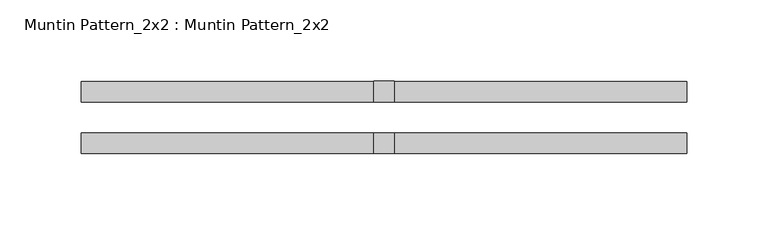
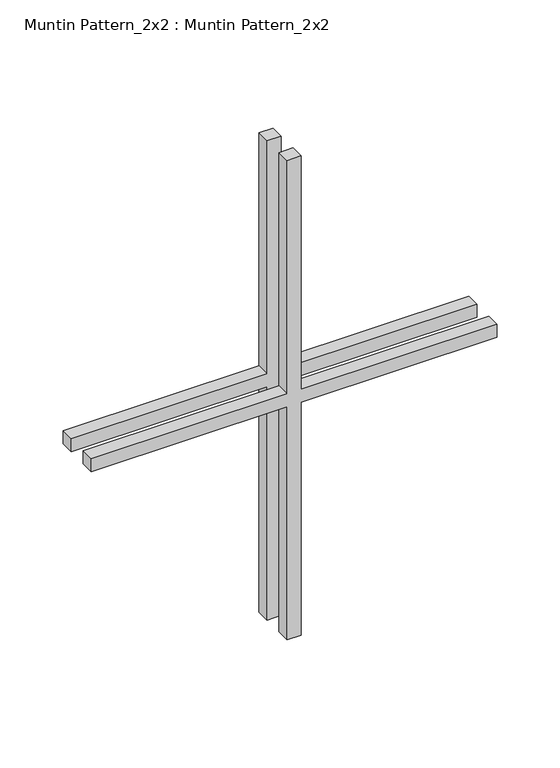
"""IFC4 building model written with IfcOpenShell, lengths in millimetres: proxy geometry, Muntin Pattern_2x2 : Muntin Pattern_2x2."""

from ifc_helpers import new_model, si_unit, frame, origin, place, context, project, spatial, polyline, outline, extrude, source, transform, mapped, element, save


def muntin_pattern_2x2_muntin_pattern_2x2_87da473c(model_context):
    return source(origin(), model_context, "Body", "SweptSolid", [
        extrude(outline(polyline([(238.125, -6.35), (238.125, -185.7375), (225.425, -185.7375), (225.425, -6.35), (0.0, -6.35), (0.0, 6.35), (225.425, 6.35), (225.425, 185.7375), (238.125, 185.7375), (238.125, 6.35), (463.55, 6.35), (463.55, -6.35), (238.125, -6.35)])), frame((0.0, 9.525, 0.0), z_axis=(0.0, 1.0, 0.0), x_axis=(0.0, 0.0, 1.0)), (0.0, 0.0, 1.0), 12.7),
        extrude(outline(polyline([(238.125, -6.35), (238.125, -185.7375), (225.425, -185.7375), (225.425, -6.35), (0.0, -6.35), (0.0, 6.35), (225.425, 6.35), (225.425, 185.7375), (238.125, 185.7375), (238.125, 6.35), (463.55, 6.35), (463.55, -6.35), (238.125, -6.35)])), frame((0.0, -22.225, 0.0), z_axis=(0.0, 1.0, 0.0), x_axis=(0.0, 0.0, 1.0)), (0.0, 0.0, 1.0), 12.7),
    ])


if __name__ == "__main__":
    model = new_model("IFC4")
    model_context = context("Model", 3, world=origin())
    ifc_project = project(units=[si_unit("LENGTHUNIT", "METRE", prefix="MILLI")], contexts=[model_context])
    site = spatial("IfcSite", under=ifc_project)
    building = spatial("IfcBuilding", under=site)
    placement = place(None, origin())
    muntin_pattern_2x2_muntin_pattern_2x2_shape = muntin_pattern_2x2_muntin_pattern_2x2_87da473c(model_context)
    element("IfcBuildingElementProxy", 1, Name="Muntin Pattern_2x2 : Muntin Pattern_2x2", ObjectType="Muntin Pattern_2x2 : Muntin Pattern_2x2", at=placement, inside=building, context=model_context, shape_type="MappedRepresentation", body=[
        mapped(muntin_pattern_2x2_muntin_pattern_2x2_shape, transform((0.0, 0.0, 0.0), x_axis=(1.0, 0.0, 0.0), y_axis=(0.0, 1.0, 0.0), z_axis=(0.0, 0.0, 1.0))),
    ])
    save(model, "model.ifc")

# Revit data of these elements
# Type "Muntin Pattern_2x2 : Muntin Pattern_2x2"
#   Width [instance default] = 4' - 0"
#   Thickness = 0' - 0 1/2"
#   Height [instance default] = 4' - 0"
#   Distance = 0' - 0 3/4"
#   Interior Material [instance default] = none
#   Exterior Material [instance default] = none
#   Default Elevation = 0
# Element 1 (IfcBuildingElementProxy, "Muntin Pattern_2x2 : Muntin Pattern_2x2")
#   Width = 1' - 2 5/8"
#   Height = 1' - 6 1/4"
#   Interior Material = Wood - Stained
#   Exterior Material = Clad - White
#   Materials on its faces: "Clad - White", "Wood - Stained"
# Materials
#   "Clad - White": class "Wood", colour RGB 0 0 0, transparency 0, Cost = 0
#   "Wood - Stained": class "Wood", colour RGB 224 178 126, transparency 0, Cost = 0
